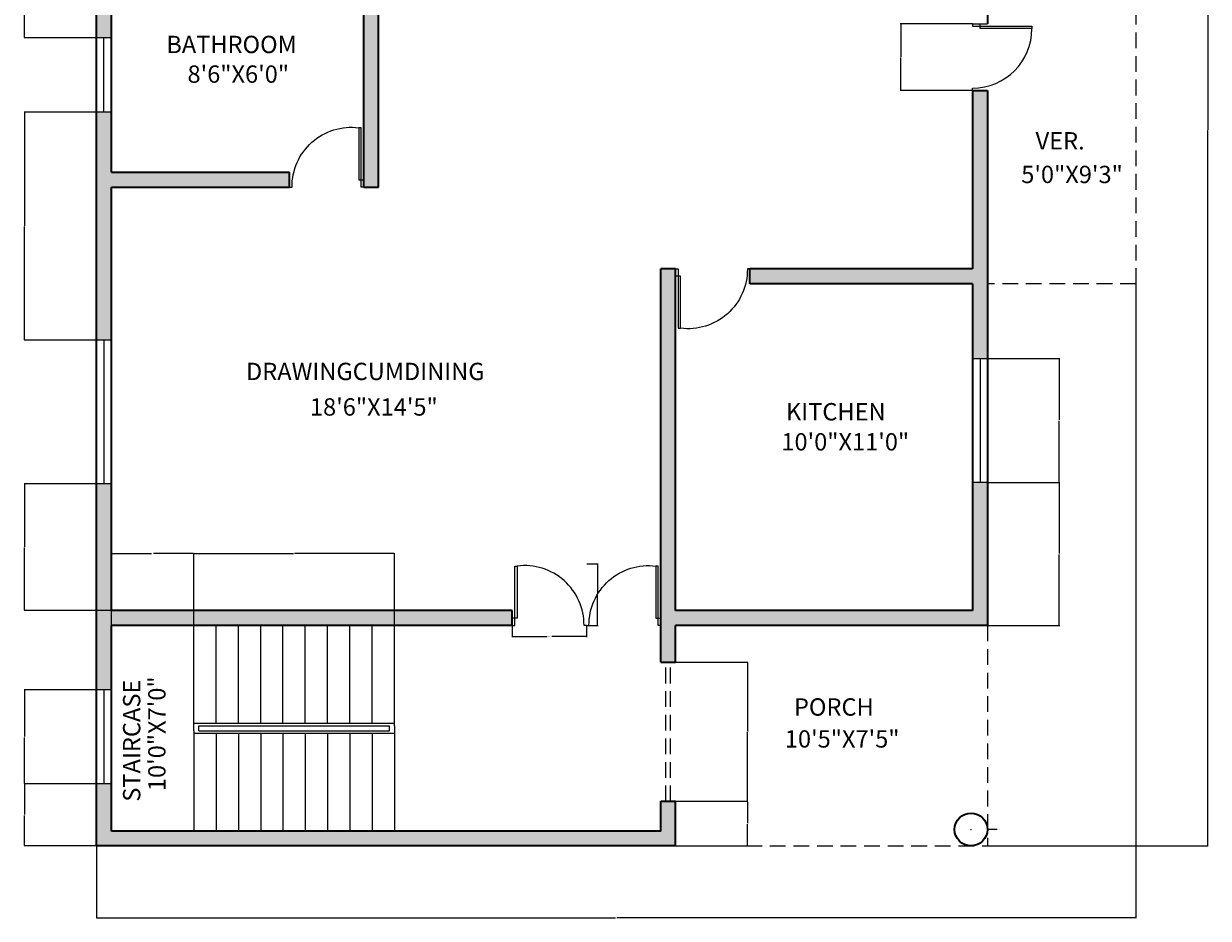
# Model space of a CAD drawing. Units: inches. Extents: x 2886 to 3365, y 1372 to 2008.
# Tile 1 of 2: x 2886 to 3365, y 1372 to 1733. Entities that reach past the tile are written whole.
import ezdxf

# ---------------------------------------------------------------- set-up
doc = ezdxf.new("R2010")
doc.units = ezdxf.units.IN
doc.linetypes.add('DASHED2', pattern=[9.525, 6.35, -3.175])
for name, color, linetype, lineweight in [('A-ANNO-DIMS', 2, 'Continuous', 18), ('A-AREA-IDEN', 50, 'Continuous', 18), ('A-COLS', 7, 'Continuous', 35), ('A-DOOR', 230, 'Continuous', 18), ('A-FLOR-OVHD', 7, 'DASHED2', 18), ('A-FLOR-STRS', 255, 'Continuous', 18), ('A-GLAZ', 7, 'Continuous', 18), ('A-WALL', 7, 'Continuous', 35)]:
    doc.layers.add(name, color=color, linetype=linetype, lineweight=lineweight)
doc.layers.add('A-WALL-PATT', color=18, linetype='Continuous', lineweight=13, true_color=0x000000)
doc.styles.get("Standard").update_dxf_attribs({"font": 'arial.ttf'})
doc.dimstyles.get("Standard").update_dxf_attribs({"dimtxt": 0.18, "dimasz": 0.18, "dimexe": 0.18, "dimexo": 0.0625, "dimgap": 0.09, "dimtad": 0, "dimtih": 1, "dimtoh": 1, "dimdec": 4, "dimzin": 0, "dimdsep": 46, "dimtxsty": 'Standard', "dimcen": 0.09, "dimadec": 0, "dimazin": 0, "dimtfac": 1, "dimtdec": 4, "dimtofl": 0, "dimtmove": 0, "dimatfit": 3, "dimfxl": 1, "dimtolj": 1, "dimtzin": 0, "dimarcsym": 0})

# ---------------------------------------------------------------- blocks, each defined once
blk = doc.blocks.new('DOOR-SWING-30IN')
for p, q in [((0, 24.19), (1, 24.19)), ((30, 24.19), (29, 24.19)), ((29, 24.19), (29, 0.19)), ((28, 0.19), (28, 21.19)), ((28, 21.19), (30, 21.19)), ((29, 0.19), (28, 0.19))]:
    blk.add_line(p, q)
blk.add_arc((25, 24), 24, 179.5504, 277.1825)
blk = doc.blocks.new('WIN-30IN')
for p, q in [((6, 30), (0, 30)), ((3, 0), (3, 30)), ((6, 0), (0, 0))]:
    blk.add_line(p, q)
blk = doc.blocks.new('WIN-58IN')
for p, q in [((6, 58), (0, 58)), ((3, 58), (3, 0)), ((6, 0), (0, 0))]:
    blk.add_line(p, q)
blk = doc.blocks.new('*D5')
at = {"layer": 'A-ANNO-DIMS', "color": 0, "lineweight": -2, "transparency": 16777216}
for p, q in [((3083.36, 1489.9), (3083.36, 1485.28)), ((3113.36, 1489.9), (3113.36, 1485.28)), ((3083.54, 1485.46), (3097.42, 1485.46)), ((3113.18, 1485.46), (3099.29, 1485.46))]:
    blk.add_line(p, q, dxfattribs=at)
at = {"layer": 'A-ANNO-DIMS', "color": 0, "transparency": 16777216}
for points in [[(3083.54, 1485.49), (3083.54, 1485.43), (3083.36, 1485.46)], [(3113.18, 1485.49), (3113.18, 1485.43), (3113.36, 1485.46)]]:
    blk.add_solid(points, dxfattribs=at)
at = {"layer": 'Defpoints', "color": 0, "transparency": 16777216}
for p in [(3083.36, 1489.96), (3113.36, 1489.96), (3083.36, 1485.46)]:
    blk.add_point(p, dxfattribs=at)
at = {"layer": 'A-ANNO-DIMS', "color": 0, "transparency": 16777216, "insert": (3098.36, 1485.46), "char_height": 0.18, "attachment_point": 5}
blk.add_mtext('\\A1;DOOR 30 TYP.', dxfattribs=at)
blk = doc.blocks.new('*D6')
at = {"layer": 'A-ANNO-DIMS', "color": 0, "lineweight": -2, "transparency": 16777216}
for p, q in [((3113.42, 1514.83), (3118.04, 1514.83)), ((3117.86, 1514.65), (3117.86, 1502.58)), ((3117.86, 1490.14), (3117.86, 1502.21)), ((3113.42, 1489.96), (3118.04, 1489.96))]:
    blk.add_line(p, q, dxfattribs=at)
at = {"layer": 'A-ANNO-DIMS', "color": 0, "transparency": 16777216}
for points in [[(3117.83, 1514.65), (3117.89, 1514.65), (3117.86, 1514.83)], [(3117.83, 1490.14), (3117.89, 1490.14), (3117.86, 1489.96)]]:
    blk.add_solid(points, dxfattribs=at)
at = {"layer": 'Defpoints', "color": 0, "transparency": 16777216}
for p in [(3113.36, 1514.83), (3113.36, 1489.96), (3117.86, 1489.96)]:
    blk.add_point(p, dxfattribs=at)
at = {"layer": 'A-ANNO-DIMS', "color": 0, "transparency": 16777216, "insert": (3117.86, 1502.4), "char_height": 0.18, "attachment_point": 5}
blk.add_mtext('\\A1;25 TYP.', dxfattribs=at)
blk = doc.blocks.new('*D13')
at = {"layer": 'A-ANNO-DIMS', "color": 0, "lineweight": -2, "transparency": 16777216}
for p, q in [((3335.36, 1627.9), (3335.36, 1371.73)), ((2915.36, 1400.9), (2915.36, 1371.73)), ((2915.54, 1371.91), (3125.07, 1371.91)), ((3335.18, 1371.91), (3125.65, 1371.91))]:
    blk.add_line(p, q, dxfattribs=at)
at = {"layer": 'A-ANNO-DIMS', "color": 0, "transparency": 16777216}
for points in [[(2915.54, 1371.94), (2915.54, 1371.88), (2915.36, 1371.91)], [(3335.18, 1371.94), (3335.18, 1371.88), (3335.36, 1371.91)]]:
    blk.add_solid(points, dxfattribs=at)
at = {"layer": 'Defpoints', "color": 0, "transparency": 16777216}
for p in [(3335.36, 1627.96), (2915.36, 1400.96), (3335.36, 1371.91)]:
    blk.add_point(p, dxfattribs=at)
at = {"layer": 'A-ANNO-DIMS', "color": 0, "transparency": 16777216, "insert": (3125.36, 1371.91), "char_height": 0.18, "attachment_point": 5}
blk.add_mtext('\\A1;420', dxfattribs=at)
blk = doc.blocks.new('*D14')
at = {"layer": 'A-ANNO-DIMS', "color": 0, "lineweight": -2, "transparency": 16777216}
for p, q in [((3275.42, 1978.96), (3364.59, 1978.96)), ((3364.41, 1978.78), (3364.41, 1690.14)), ((3364.41, 1401.14), (3364.41, 1689.78)), ((3275.42, 1400.96), (3364.59, 1400.96))]:
    blk.add_line(p, q, dxfattribs=at)
at = {"layer": 'A-ANNO-DIMS', "color": 0, "transparency": 16777216}
for points in [[(3364.38, 1978.78), (3364.44, 1978.78), (3364.41, 1978.96)], [(3364.38, 1401.14), (3364.44, 1401.14), (3364.41, 1400.96)]]:
    blk.add_solid(points, dxfattribs=at)
at = {"layer": 'Defpoints', "color": 0, "transparency": 16777216}
for p in [(3275.36, 1978.96), (3364.41, 1978.96), (3275.36, 1400.96)]:
    blk.add_point(p, dxfattribs=at)
at = {"layer": 'A-ANNO-DIMS', "color": 0, "transparency": 16777216, "insert": (3364.41, 1689.96), "char_height": 0.18, "attachment_point": 5}
blk.add_mtext('\\A1;578', dxfattribs=at)
blk = doc.blocks.new('*D16')
at = {"layer": 'A-ANNO-DIMS', "color": 0, "lineweight": -2, "transparency": 16777216}
for p, q in [((2915.29, 1425.98), (2886.13, 1425.98)), ((2886.31, 1425.8), (2886.31, 1413.65)), ((2886.31, 1401.14), (2886.31, 1413.29)), ((2915.29, 1400.96), (2886.13, 1400.96))]:
    blk.add_line(p, q, dxfattribs=at)
at = {"layer": 'A-ANNO-DIMS', "color": 0, "transparency": 16777216}
for points in [[(2886.28, 1425.8), (2886.34, 1425.8), (2886.31, 1425.98)], [(2886.28, 1401.14), (2886.34, 1401.14), (2886.31, 1400.96)]]:
    blk.add_solid(points, dxfattribs=at)
at = {"layer": 'Defpoints', "color": 0, "transparency": 16777216}
for p in [(2886.31, 1425.98), (2915.36, 1425.98), (2915.36, 1400.96)]:
    blk.add_point(p, dxfattribs=at)
at = {"layer": 'A-ANNO-DIMS', "color": 0, "transparency": 16777216, "insert": (2886.31, 1413.47), "char_height": 0.18, "attachment_point": 5}
blk.add_mtext('\\A1;25.014', dxfattribs=at)
blk = doc.blocks.new('*D17')
at = {"layer": 'A-ANNO-DIMS', "color": 0, "lineweight": -2, "transparency": 16777216}
for p, q in [((2915.29, 1463.98), (2886.13, 1463.98)), ((2886.31, 1463.8), (2886.31, 1445.16)), ((2886.31, 1426.16), (2886.31, 1444.79)), ((2915.29, 1425.98), (2886.13, 1425.98))]:
    blk.add_line(p, q, dxfattribs=at)
at = {"layer": 'A-ANNO-DIMS', "color": 0, "transparency": 16777216}
for points in [[(2886.28, 1463.8), (2886.34, 1463.8), (2886.31, 1463.98)], [(2886.28, 1426.16), (2886.34, 1426.16), (2886.31, 1425.98)]]:
    blk.add_solid(points, dxfattribs=at)
at = {"layer": 'Defpoints', "color": 0, "transparency": 16777216}
for p in [(2886.31, 1463.98), (2915.36, 1463.98), (2915.36, 1425.98)]:
    blk.add_point(p, dxfattribs=at)
at = {"layer": 'A-ANNO-DIMS', "color": 0, "transparency": 16777216, "insert": (2886.31, 1444.98), "char_height": 0.18, "attachment_point": 5}
blk.add_mtext('\\A1;38', dxfattribs=at)
blk = doc.blocks.new('*D18')
at = {"layer": 'A-ANNO-DIMS', "color": 0, "lineweight": -2, "transparency": 16777216}
for p, q in [((2915.29, 1547.19), (2886.13, 1547.19)), ((2886.31, 1547.01), (2886.31, 1521.76)), ((2886.31, 1496.14), (2886.31, 1521.4)), ((2921.29, 1495.96), (2886.13, 1495.96))]:
    blk.add_line(p, q, dxfattribs=at)
at = {"layer": 'A-ANNO-DIMS', "color": 0, "transparency": 16777216}
for points in [[(2886.28, 1547.01), (2886.34, 1547.01), (2886.31, 1547.19)], [(2886.28, 1496.14), (2886.34, 1496.14), (2886.31, 1495.96)]]:
    blk.add_solid(points, dxfattribs=at)
at = {"layer": 'Defpoints', "color": 0, "transparency": 16777216}
for p in [(2886.31, 1547.19), (2915.36, 1547.19), (2921.36, 1495.96)]:
    blk.add_point(p, dxfattribs=at)
at = {"layer": 'A-ANNO-DIMS', "color": 0, "transparency": 16777216, "insert": (2886.31, 1521.58), "char_height": 0.18, "attachment_point": 5}
blk.add_mtext('\\A1;51.23', dxfattribs=at)
blk = doc.blocks.new('*D19')
at = {"layer": 'A-ANNO-DIMS', "color": 0, "lineweight": -2, "transparency": 16777216}
for p, q in [((2915.29, 1697.2), (2886.13, 1697.2)), ((2886.31, 1697.02), (2886.31, 1651.38)), ((2886.31, 1605.37), (2886.31, 1651.02)), ((2915.29, 1605.19), (2886.13, 1605.19))]:
    blk.add_line(p, q, dxfattribs=at)
at = {"layer": 'A-ANNO-DIMS', "color": 0, "transparency": 16777216}
for points in [[(2886.28, 1697.02), (2886.34, 1697.02), (2886.31, 1697.2)], [(2886.28, 1605.37), (2886.34, 1605.37), (2886.31, 1605.19)]]:
    blk.add_solid(points, dxfattribs=at)
at = {"layer": 'Defpoints', "color": 0, "transparency": 16777216}
for p in [(2886.31, 1697.2), (2915.36, 1697.2), (2915.36, 1605.19)]:
    blk.add_point(p, dxfattribs=at)
at = {"layer": 'A-ANNO-DIMS', "color": 0, "transparency": 16777216, "insert": (2886.31, 1651.2), "char_height": 0.18, "attachment_point": 5}
blk.add_mtext('\\A1;92', dxfattribs=at)
blk = doc.blocks.new('*D20')
at = {"layer": 'A-ANNO-DIMS', "color": 0, "lineweight": -2, "transparency": 16777216}
for p, q in [((2915.29, 1775.81), (2886.13, 1775.81)), ((2886.31, 1775.63), (2886.31, 1751.69)), ((2886.31, 1727.38), (2886.31, 1751.32)), ((2915.29, 1727.2), (2886.13, 1727.2))]:
    blk.add_line(p, q, dxfattribs=at)
at = {"layer": 'A-ANNO-DIMS', "color": 0, "transparency": 16777216}
for points in [[(2886.28, 1775.63), (2886.34, 1775.63), (2886.31, 1775.81)], [(2886.28, 1727.38), (2886.34, 1727.38), (2886.31, 1727.2)]]:
    blk.add_solid(points, dxfattribs=at)
at = {"layer": 'Defpoints', "color": 0, "transparency": 16777216}
for p in [(2886.31, 1775.81), (2915.36, 1775.81), (2915.36, 1727.2)]:
    blk.add_point(p, dxfattribs=at)
at = {"layer": 'A-ANNO-DIMS', "color": 0, "transparency": 16777216, "insert": (2886.31, 1751.5), "char_height": 0.18, "attachment_point": 5}
blk.add_mtext('\\A1;48.61', dxfattribs=at)
blk = doc.blocks.new('*D21')
at = {"layer": 'A-ANNO-DIMS', "color": 0, "lineweight": -2, "transparency": 16777216}
for p, q in [((3275.42, 1547.77), (3304.59, 1547.77)), ((3304.41, 1547.59), (3304.41, 1519.05)), ((3304.41, 1490.14), (3304.41, 1518.69)), ((3275.42, 1489.96), (3304.59, 1489.96))]:
    blk.add_line(p, q, dxfattribs=at)
at = {"layer": 'A-ANNO-DIMS', "color": 0, "transparency": 16777216}
for points in [[(3304.38, 1547.59), (3304.44, 1547.59), (3304.41, 1547.77)], [(3304.38, 1490.14), (3304.44, 1490.14), (3304.41, 1489.96)]]:
    blk.add_solid(points, dxfattribs=at)
at = {"layer": 'Defpoints', "color": 0, "transparency": 16777216}
for p in [(3275.36, 1547.77), (3275.36, 1489.96), (3304.41, 1489.96)]:
    blk.add_point(p, dxfattribs=at)
at = {"layer": 'A-ANNO-DIMS', "color": 0, "transparency": 16777216, "insert": (3304.41, 1518.87), "char_height": 0.18, "attachment_point": 5}
blk.add_mtext('\\A1;57.81', dxfattribs=at)
blk = doc.blocks.new('*D22')
at = {"layer": 'A-ANNO-DIMS', "color": 0, "lineweight": -2, "transparency": 16777216}
for p, q in [((3275.42, 1597.77), (3304.59, 1597.77)), ((3304.41, 1597.59), (3304.41, 1572.95)), ((3304.41, 1547.95), (3304.41, 1572.59)), ((3275.42, 1547.77), (3304.59, 1547.77))]:
    blk.add_line(p, q, dxfattribs=at)
at = {"layer": 'A-ANNO-DIMS', "color": 0, "transparency": 16777216}
for points in [[(3304.38, 1597.59), (3304.44, 1597.59), (3304.41, 1597.77)], [(3304.38, 1547.95), (3304.44, 1547.95), (3304.41, 1547.77)]]:
    blk.add_solid(points, dxfattribs=at)
at = {"layer": 'Defpoints', "color": 0, "transparency": 16777216}
for p in [(3275.36, 1597.77), (3275.36, 1547.77), (3304.41, 1547.77)]:
    blk.add_point(p, dxfattribs=at)
at = {"layer": 'A-ANNO-DIMS', "color": 0, "transparency": 16777216, "insert": (3304.41, 1572.77), "char_height": 0.18, "attachment_point": 5}
blk.add_mtext('\\A1;50', dxfattribs=at)
blk = doc.blocks.new('*D24')
at = {"layer": 'A-ANNO-DIMS', "color": 0, "lineweight": -2, "transparency": 16777216}
for p, q in [((3269.29, 1732.96), (3240.13, 1732.96)), ((3240.31, 1732.78), (3240.31, 1719.64)), ((3240.31, 1706.14), (3240.31, 1719.28)), ((3269.29, 1705.96), (3240.13, 1705.96))]:
    blk.add_line(p, q, dxfattribs=at)
at = {"layer": 'A-ANNO-DIMS', "color": 0, "transparency": 16777216}
for points in [[(3240.28, 1732.78), (3240.34, 1732.78), (3240.31, 1732.96)], [(3240.28, 1706.14), (3240.34, 1706.14), (3240.31, 1705.96)]]:
    blk.add_solid(points, dxfattribs=at)
at = {"layer": 'Defpoints', "color": 0, "transparency": 16777216}
for p in [(3240.31, 1732.96), (3269.36, 1732.96), (3269.36, 1705.96)]:
    blk.add_point(p, dxfattribs=at)
at = {"layer": 'A-ANNO-DIMS', "color": 0, "transparency": 16777216, "insert": (3240.31, 1719.46), "char_height": 0.18, "attachment_point": 5}
blk.add_mtext('\\A1;27', dxfattribs=at)
blk = doc.blocks.new('*D26')
at = {"layer": 'A-ANNO-DIMS', "color": 0, "lineweight": -2, "transparency": 16777216}
for p, q in [((2921.36, 1490.02), (2921.36, 1519.19)), ((2921.54, 1519.01), (2937.64, 1519.01)), ((2954.53, 1519.01), (2938.43, 1519.01)), ((2954.71, 1490.02), (2954.71, 1519.19))]:
    blk.add_line(p, q, dxfattribs=at)
at = {"layer": 'A-ANNO-DIMS', "color": 0, "transparency": 16777216}
for points in [[(2921.54, 1519.04), (2921.54, 1518.98), (2921.36, 1519.01)], [(2954.53, 1519.04), (2954.53, 1518.98), (2954.71, 1519.01)]]:
    blk.add_solid(points, dxfattribs=at)
at = {"layer": 'Defpoints', "color": 0, "transparency": 16777216}
for p in [(2954.71, 1519.01), (2921.36, 1489.96), (2954.71, 1489.96)]:
    blk.add_point(p, dxfattribs=at)
at = {"layer": 'A-ANNO-DIMS', "color": 0, "transparency": 16777216, "insert": (2938.03, 1519.01), "char_height": 0.18, "attachment_point": 5}
blk.add_mtext('\\A1;33.35', dxfattribs=at)
blk = doc.blocks.new('*D27')
at = {"layer": 'A-ANNO-DIMS', "color": 0, "lineweight": -2, "transparency": 16777216}
for p, q in [((2954.71, 1490.02), (2954.71, 1519.19)), ((2954.89, 1519.01), (2995.01, 1519.01)), ((3035.53, 1519.01), (2995.41, 1519.01)), ((3035.71, 1490.02), (3035.71, 1519.19))]:
    blk.add_line(p, q, dxfattribs=at)
at = {"layer": 'A-ANNO-DIMS', "color": 0, "transparency": 16777216}
for points in [[(2954.89, 1519.04), (2954.89, 1518.98), (2954.71, 1519.01)], [(3035.53, 1519.04), (3035.53, 1518.98), (3035.71, 1519.01)]]:
    blk.add_solid(points, dxfattribs=at)
at = {"layer": 'Defpoints', "color": 0, "transparency": 16777216}
for p in [(3035.71, 1519.01), (2954.71, 1489.96), (3035.71, 1489.96)]:
    blk.add_point(p, dxfattribs=at)
at = {"layer": 'A-ANNO-DIMS', "color": 0, "transparency": 16777216, "insert": (2995.21, 1519.01), "char_height": 0.18, "attachment_point": 5}
blk.add_mtext('\\A1;81', dxfattribs=at)
blk = doc.blocks.new('*D28')
at = {"layer": 'A-ANNO-DIMS', "color": 0, "lineweight": -2, "transparency": 16777216}
for p, q in [((3149.42, 1475.2), (3178.59, 1475.2)), ((3178.41, 1475.02), (3178.41, 1447.27)), ((3178.41, 1419.14), (3178.41, 1446.9)), ((3149.42, 1418.96), (3178.59, 1418.96))]:
    blk.add_line(p, q, dxfattribs=at)
at = {"layer": 'A-ANNO-DIMS', "color": 0, "transparency": 16777216}
for points in [[(3178.38, 1475.02), (3178.44, 1475.02), (3178.41, 1475.2)], [(3178.38, 1419.14), (3178.44, 1419.14), (3178.41, 1418.96)]]:
    blk.add_solid(points, dxfattribs=at)
at = {"layer": 'Defpoints', "color": 0, "transparency": 16777216}
for p in [(3149.36, 1475.2), (3149.36, 1418.96), (3178.41, 1418.96)]:
    blk.add_point(p, dxfattribs=at)
at = {"layer": 'A-ANNO-DIMS', "color": 0, "transparency": 16777216, "insert": (3178.41, 1447.08), "char_height": 0.18, "attachment_point": 5}
blk.add_mtext('\\A1;56.24', dxfattribs=at)
blk = doc.blocks.new('*D29')
at = {"layer": 'A-ANNO-DIMS', "color": 0, "lineweight": -2, "transparency": 16777216}
for p, q in [((3149.42, 1418.96), (3178.59, 1418.96)), ((3178.41, 1418.78), (3178.41, 1410.14)), ((3178.41, 1401.14), (3178.41, 1409.78)), ((3149.42, 1400.96), (3178.59, 1400.96))]:
    blk.add_line(p, q, dxfattribs=at)
at = {"layer": 'A-ANNO-DIMS', "color": 0, "transparency": 16777216}
for points in [[(3178.38, 1418.78), (3178.44, 1418.78), (3178.41, 1418.96)], [(3178.38, 1401.14), (3178.44, 1401.14), (3178.41, 1400.96)]]:
    blk.add_solid(points, dxfattribs=at)
at = {"layer": 'Defpoints', "color": 0, "transparency": 16777216}
for p in [(3149.36, 1418.96), (3149.36, 1400.96), (3178.41, 1400.96)]:
    blk.add_point(p, dxfattribs=at)
at = {"layer": 'A-ANNO-DIMS', "color": 0, "transparency": 16777216, "insert": (3178.41, 1409.96), "char_height": 0.18, "attachment_point": 5}
blk.add_mtext('\\A1;18', dxfattribs=at)
blk = doc.blocks.new('*D30')
at = {"layer": 'A-ANNO-DIMS', "color": 0, "lineweight": -2, "transparency": 16777216}
for p, q in [((3268.64, 1407.59), (3268.82, 1407.59)), ((3268.73, 1407.5), (3268.73, 1407.68)), ((3279.34, 1407.59), (3275.54, 1407.59))]:
    blk.add_line(p, q, dxfattribs=at)
at = {"layer": 'A-ANNO-DIMS', "color": 0, "transparency": 16777216}
blk.add_solid([(3275.54, 1407.62), (3275.54, 1407.56), (3275.36, 1407.59)], dxfattribs=at)
at = {"layer": 'Defpoints', "color": 0, "transparency": 16777216}
for p in [(3262.1, 1407.59), (3275.36, 1407.59)]:
    blk.add_point(p, dxfattribs=at)
at = {"layer": 'A-ANNO-DIMS', "color": 0, "transparency": 16777216, "insert": (3279.83, 1407.59), "char_height": 0.18, "attachment_point": 5}
blk.add_mtext('\\A1;∅13.26', dxfattribs=at)

msp = doc.modelspace()

# ---------------------------------------------------------------- hatches: boundary and pattern name
at = {"layer": 'A-WALL-PATT'}
h = msp.add_hatch(color=256, dxfattribs=at)
h.dxf.hatch_style = 1
h.paths.add_polyline_path([(3059.3575, 1840.9624), (3023.3575, 1840.9624), (3023.3575, 1750.9624), (2921.3575, 1750.9624), (2921.3575, 1775.8094), (2915.3575, 1775.8094), (2915.3575, 1727.2), (2921.3575, 1727.2), (2921.3575, 1744.9624), (3023.3575, 1744.9624), (3023.3575, 1666.9624), (3029.3575, 1666.9624), (3029.3575, 1834.9624), (3059.3575, 1834.9624)])
h = msp.add_hatch(color=256, dxfattribs=at)
h.dxf.hatch_style = 1
h.paths.add_polyline_path([(3275.3575, 1705.9624), (3269.3575, 1705.9624), (3269.3575, 1633.9624), (3179.3575, 1633.9624), (3179.3575, 1627.9624), (3269.3575, 1627.9624), (3269.3575, 1597.7716), (3275.3575, 1597.7716)])
h = msp.add_hatch(color=256, dxfattribs=at)
h.dxf.hatch_style = 1
h.paths.add_polyline_path([(2993.3575, 1672.9624), (2921.3575, 1672.9624), (2921.3575, 1697.2), (2915.3575, 1697.2), (2915.3575, 1605.1944), (2921.3575, 1605.1944), (2921.3575, 1666.9624), (2993.3575, 1666.9624)])
h = msp.add_hatch(color=256, dxfattribs=at)
h.dxf.hatch_style = 1
h.paths.add_polyline_path([(3149.3575, 1633.9624), (3143.3575, 1633.9624), (3143.3575, 1475.2041), (3149.3575, 1475.2041), (3149.3575, 1489.9624), (3275.3575, 1489.9624), (3275.3575, 1547.7716), (3269.3575, 1547.7716), (3269.3575, 1495.9624), (3149.3575, 1495.9624)])
h = msp.add_hatch(color=256, dxfattribs=at)
h.dxf.hatch_style = 1
h.paths.add_polyline_path([(3083.3575, 1495.9624), (2921.3575, 1495.9624), (2921.3575, 1547.1944), (2915.3575, 1547.1944), (2915.3575, 1463.9764), (2921.3575, 1463.9764), (2921.3575, 1489.9624), (3083.3575, 1489.9624)])
h = msp.add_hatch(color=256, dxfattribs=at)
h.dxf.hatch_style = 1
h.paths.add_polyline_path([(3149.3575, 1418.9624), (3143.3575, 1418.9624), (3143.3575, 1406.9624), (2921.3575, 1406.9624), (2921.3575, 1425.9764), (2915.3575, 1425.9764), (2915.3575, 1400.9624), (3149.3575, 1400.9624)])

# ---------------------------------------------------------------- linework, layer by layer
at = {"layer": 'A-COLS'}
msp.add_circle((3268.7272, 1407.5927), 6.6303, dxfattribs=at)
at = {"layer": 'A-DOOR'}
for p, q in [((3269.3575, 1732.9624), (3275.3575, 1732.9624)), ((3269.3575, 1732.9624), (3269.3575, 1731.9624)), ((3272.3575, 1730.9624), (3272.3575, 1732.9624)), ((3269.3575, 1731.9624), (3293.3575, 1731.9624)), ((3293.3575, 1730.9624), (3272.3575, 1730.9624)), ((3293.3575, 1731.9624), (3293.3575, 1730.9624)), ((3269.3575, 1705.9624), (3269.3575, 1706.9624))]:
    msp.add_line(p, q, dxfattribs=at)
msp.add_arc((3269.3575, 1730.9624), 24, 270, 0, dxfattribs=at)
at = {"layer": 'A-FLOR-OVHD'}
for p, q in [((3335.3575, 1738.9624), (3335.3575, 1627.9624)), ((3335.3575, 1627.9624), (3275.3575, 1627.9624)), ((3275.3575, 1489.9624), (3275.3575, 1400.9624)), ((3145.3575, 1418.9624), (3145.3575, 1475.2041)), ((3147.3575, 1418.9624), (3147.3575, 1475.2041)), ((3149.3575, 1400.9624), (3275.3575, 1400.9624))]:
    msp.add_line(p, q, dxfattribs=at)
at = {"layer": 'A-FLOR-STRS'}
for p, q in [((2954.7074, 1449.4624), (2954.7074, 1489.9624)), ((2963.7074, 1450.4624), (2963.7074, 1489.9624)), ((2972.7074, 1450.4624), (2972.7074, 1489.9624)), ((2981.7074, 1450.4624), (2981.7074, 1489.9624)), ((2990.7074, 1450.4624), (2990.7074, 1489.9624)), ((2999.7074, 1450.4624), (2999.7074, 1489.9624)), ((3008.7074, 1450.4624), (3008.7074, 1489.9624)), ((3017.7074, 1450.4624), (3017.7074, 1489.9624)), ((3026.7074, 1450.4624), (3026.7074, 1489.9624)), ((3035.7074, 1449.4624), (3035.7074, 1489.9624)), ((2954.7074, 1450.4624), (3035.7074, 1450.4624)), ((2954.7074, 1447.4624), (2954.7074, 1449.4624)), ((2954.7074, 1447.4624), (2954.7074, 1406.9624)), ((2954.7074, 1446.4624), (3035.7074, 1446.4624)), ((2956.7074, 1449.4624), (3033.7074, 1449.4624)), ((2956.7074, 1447.4624), (2956.7074, 1449.4624)), ((2956.7074, 1447.4624), (3033.7074, 1447.4624)), ((2963.7074, 1446.4624), (2963.7074, 1406.9624)), ((2972.7074, 1446.4624), (2972.7074, 1406.9624)), ((2981.7074, 1446.4624), (2981.7074, 1406.9624)), ((2990.7074, 1446.4624), (2990.7074, 1406.9624)), ((2999.7074, 1446.4624), (2999.7074, 1406.9624)), ((3008.7074, 1446.4624), (3008.7074, 1406.9624)), ((3017.7074, 1446.4624), (3017.7074, 1406.9624)), ((3026.7074, 1446.4624), (3026.7074, 1406.9624)), ((3033.7074, 1447.4624), (3033.7074, 1449.4624)), ((3035.7074, 1449.4624), (3035.7074, 1406.9624))]:
    msp.add_line(p, q, dxfattribs=at)
at = {"layer": 'A-GLAZ'}
for p, q in [((3269.3575, 1597.7716), (3275.3575, 1597.7716)), ((3272.3575, 1597.7716), (3272.3575, 1547.7716)), ((3269.3575, 1547.7716), (3275.3575, 1547.7716)), ((2921.3575, 1463.9764), (2915.3575, 1463.9764)), ((2918.3575, 1463.9764), (2918.3575, 1425.9764)), ((2921.3575, 1425.9764), (2915.3575, 1425.9764))]:
    msp.add_line(p, q, dxfattribs=at)
at = {"layer": 'A-WALL'}
for p, q in [((3029.3575, 1666.9624), (3029.3575, 1834.9624)), ((2921.3575, 1672.9624), (2921.3575, 1744.9624)), ((3023.3575, 1666.9624), (3023.3575, 1744.9624)), ((3269.3575, 1705.9624), (3269.3575, 1633.9624)), ((3269.3575, 1705.9624), (3275.3575, 1705.9624)), ((2921.3575, 1672.9624), (2993.3575, 1672.9624)), ((2993.3575, 1666.9624), (2993.3575, 1672.9624)), ((2921.3575, 1666.9624), (2993.3575, 1666.9624)), ((2921.3575, 1495.9624), (2921.3575, 1666.9624)), ((3023.3575, 1666.9624), (3029.3575, 1666.9624)), ((3149.3575, 1633.9624), (3143.3575, 1633.9624)), ((3143.3575, 1475.2041), (3143.3575, 1633.9624)), ((3149.3575, 1495.9624), (3149.3575, 1633.9624)), ((3269.3575, 1633.9624), (3179.3575, 1633.9624)), ((3179.3575, 1627.9624), (3179.3575, 1633.9624)), ((3269.3575, 1627.9624), (3179.3575, 1627.9624)), ((3269.3575, 1627.9624), (3269.3575, 1495.9624)), ((3083.3575, 1495.9624), (2921.3575, 1495.9624)), ((3083.3575, 1489.9624), (3083.3575, 1495.9624)), ((3269.3575, 1495.9624), (3149.3575, 1495.9624)), ((2921.3575, 1406.9624), (2921.3575, 1489.9624)), ((3083.3575, 1489.9624), (2921.3575, 1489.9624)), ((3275.3575, 1489.9624), (3149.3575, 1489.9624)), ((3149.3575, 1475.2041), (3149.3575, 1489.9624)), ((3143.3575, 1475.2041), (3149.3575, 1475.2041)), ((3143.3575, 1406.9624), (3143.3575, 1418.9624)), ((3143.3575, 1418.9624), (3149.3575, 1418.9624)), ((3149.3575, 1400.9624), (3149.3575, 1418.9624)), ((3143.3575, 1406.9624), (2921.3575, 1406.9624))]:
    msp.add_line(p, q, dxfattribs=at)
for points in [[(3149.3575, 1400.9624), (2915.3575, 1400.9624), (2915.3575, 1978.9624), (3275.3575, 1978.9624), (3275.3575, 1732.9624)], [(3275.3575, 1705.9624), (3275.3575, 1489.9624)]]:
    msp.add_lwpolyline(points, dxfattribs=at)

# ---------------------------------------------------------------- block references
at = {"layer": 'A-DOOR', "extrusion": (0, 0, -1), "zscale": -1, "rotation": 180}
for p in [(-2993.357, 1691.1498), (-3113.357, 1514.1498)]:
    msp.add_blockref('DOOR-SWING-30IN', p, dxfattribs=at)
at = {"layer": 'A-DOOR', "extrusion": (0, 0, -1), "zscale": -1}
msp.add_blockref('DOOR-SWING-30IN', (-3179.358, 1609.775), dxfattribs=at)
at = {"layer": 'A-DOOR', "rotation": 180}
msp.add_blockref('DOOR-SWING-30IN', (3113.358, 1514.1498), dxfattribs=at)
at = {"layer": 'A-GLAZ'}
for name, p in [('WIN-30IN', (2915.357, 1697.1996)), ('WIN-58IN', (2915.357, 1547.194))]:
    msp.add_blockref(name, p, dxfattribs=at)

# ---------------------------------------------------------------- texts
at = {"layer": 'A-AREA-IDEN'}
for tag, p in [('BATHROOM', (2943.5612, 1721.0861)), ('8\'6"X6\'0"', (2952.1212, 1709.1123)), ('VER.', (3294.8138, 1682.1795)), ('5\'0"X9\'3"', (3289.0294, 1668.6007)), ('DRAWINGCUMDINING', (2975.7607, 1589.05)), ('18\'6"X14\'5"', (3001.6013, 1574.7064)), ('KITCHEN', (3193.9567, 1572.7816)), ('10\'0"X11\'0"', (3192.091, 1560.6272)), ('PORCH', (3197.1819, 1453.5543)), ('10\'5"X7\'5"', (3193.496, 1440.6649))]:
    msp.add_attdef(tag, p, '', height=7, dxfattribs=at)
for tag, p in [('STAIRCASE', (2933.065, 1418.8134)), ('10\'0"X7\'0"', (2943.25, 1423.0766))]:
    msp.add_attdef(tag, p, '', height=7, rotation=90, dxfattribs=at)

# ---------------------------------------------------------------- dimensions: what is measured, and where the dimension line sits
at = {"layer": 'A-ANNO-DIMS'}
for base, p1, p2, angle, override, picture, middle in [((3364.4075, 1978.9624), (3275.3575, 1400.9624), (3275.3575, 1978.9624), 90, {"dimdec": 0, "dimlfac": 1, "dimrnd": 0, "dimzin": 0, "dimdsep": 46, "dimlunit": 2}, '*D14', (3364.4075, 1689.9624)), ((2886.3075, 1775.8094), (2915.3575, 1727.2), (2915.3575, 1775.8094), 90, {"dimdec": 2, "dimlfac": 1, "dimrnd": 0, "dimzin": 0, "dimdsep": 46, "dimlunit": 2}, '*D20', (2886.3075, 1751.5047)), ((3240.3075, 1732.9624), (3269.3575, 1705.9624), (3269.3575, 1732.9624), 90, {"dimdec": 0, "dimlfac": 1, "dimrnd": 0, "dimzin": 0, "dimdsep": 46, "dimlunit": 2}, '*D24', (3240.3075, 1719.4624)), ((2886.3075, 1697.2), (2915.3575, 1605.1944), (2915.3575, 1697.2), 90, {"dimdec": 0, "dimlfac": 1, "dimrnd": 0, "dimzin": 0, "dimdsep": 46, "dimlunit": 2}, '*D19', (2886.3075, 1651.1972)), ((3304.4075, 1547.7716), (3275.3575, 1597.7716), (3275.3575, 1547.7716), 270, {"dimdec": 0, "dimlfac": 1, "dimrnd": 0, "dimzin": 0, "dimdsep": 46, "dimlunit": 2}, '*D22', (3304.4075, 1572.7716)), ((2886.3075, 1547.1944), (2921.3575, 1495.9624), (2915.3575, 1547.1944), 90, {"dimdec": 2, "dimlfac": 1, "dimrnd": 0, "dimzin": 0, "dimdsep": 46, "dimlunit": 2}, '*D18', (2886.3075, 1521.5784)), ((3304.4075, 1489.9624), (3275.3575, 1547.7716), (3275.3575, 1489.9624), 270, {"dimdec": 2, "dimlfac": 1, "dimrnd": 0, "dimzin": 0, "dimdsep": 46, "dimlunit": 2}, '*D21', (3304.4075, 1518.867)), ((3178.4075, 1418.9624), (3149.3575, 1475.2041), (3149.3575, 1418.9624), 270, {"dimdec": 2, "dimlfac": 1, "dimrnd": 0, "dimzin": 0, "dimdsep": 46, "dimlunit": 2}, '*D28', (3178.4075, 1447.0832)), ((2886.3075, 1463.9764), (2915.3575, 1425.9764), (2915.3575, 1463.9764), 90, {"dimdec": 0, "dimlfac": 1, "dimrnd": 0, "dimzin": 0, "dimdsep": 46, "dimlunit": 2}, '*D17', (2886.3075, 1444.9764)), ((2886.3075, 1425.9764), (2915.3575, 1400.9624), (2915.3575, 1425.9764), 90, {"dimdec": 3, "dimlfac": 1, "dimrnd": 0, "dimzin": 0, "dimdsep": 46, "dimlunit": 2}, '*D16', (2886.3075, 1413.4694)), ((3178.4075, 1400.9624), (3149.3575, 1418.9624), (3149.3575, 1400.9624), 270, {"dimdec": 0, "dimlfac": 1, "dimrnd": 0, "dimzin": 0, "dimdsep": 46, "dimlunit": 2}, '*D29', (3178.4075, 1409.9624))]:
    dim = msp.add_linear_dim(base=base, p1=p1, p2=p2, angle=angle, dimstyle='Standard', override=override, dxfattribs=at)
    dim.commit()
    dim.dimension.update_dxf_attribs({"geometry": picture, "text_midpoint": middle})
for base, p1, p2, override, picture, middle in [((3335.3575, 1371.9124), (2915.3575, 1400.9624), (3335.3575, 1627.9624), {"dimdec": 0, "dimlfac": 1, "dimrnd": 0, "dimzin": 0, "dimdsep": 46, "dimlunit": 2}, '*D13', (3125.3575, 1371.9124)), ((2954.7074, 1519.0124), (2921.3575, 1489.9624), (2954.7074, 1489.9624), {"dimdec": 2, "dimlfac": 1, "dimrnd": 0, "dimzin": 0, "dimdsep": 46, "dimlunit": 2}, '*D26', (2938.0324, 1519.0124)), ((3035.7074, 1519.0124), (2954.7074, 1489.9624), (3035.7074, 1489.9624), {"dimdec": 0, "dimlfac": 1, "dimrnd": 0, "dimzin": 0, "dimdsep": 46, "dimlunit": 2}, '*D27', (2995.2074, 1519.0124))]:
    dim = msp.add_linear_dim(base=base, p1=p1, p2=p2, dimstyle='Standard', override=override, dxfattribs=at)
    dim.commit()
    dim.dimension.update_dxf_attribs({"geometry": picture, "text_midpoint": middle})
for base, p1, p2, angle, text, picture, middle in [((3117.8575, 1489.9624), (3113.3575, 1514.8278), (3113.3575, 1489.9624), 270, '<> TYP.', '*D6', (3117.8575, 1502.3951)), ((3083.3575, 1485.4624), (3113.3575, 1489.9624), (3083.3575, 1489.9624), 180, 'DOOR <> TYP.', '*D5', (3098.3575, 1485.4624))]:
    dim = msp.add_linear_dim(base=base, p1=p1, p2=p2, angle=angle, text=text, dimstyle='Standard', override={"dimdec": 0, "dimlfac": 1, "dimrnd": 0, "dimzin": 0, "dimdsep": 46, "dimlunit": 2}, dxfattribs=at)
    dim.commit()
    dim.dimension.update_dxf_attribs({"geometry": picture, "text_midpoint": middle})
dim = msp.add_diameter_dim_2p(p1=(3262.0969, 1407.5924), p2=(3275.3575, 1407.593), dimstyle='Standard', override={"dimdec": 2, "dimlfac": 1, "dimrnd": 0, "dimzin": 0, "dimdsep": 46, "dimlunit": 2}, dxfattribs=at)
dim.commit()
dim.dimension.update_dxf_attribs({"geometry": '*D30', "text_midpoint": (3279.3357, 1407.5932), "dimtype": 163})

doc.saveas('drawing.dxf')
